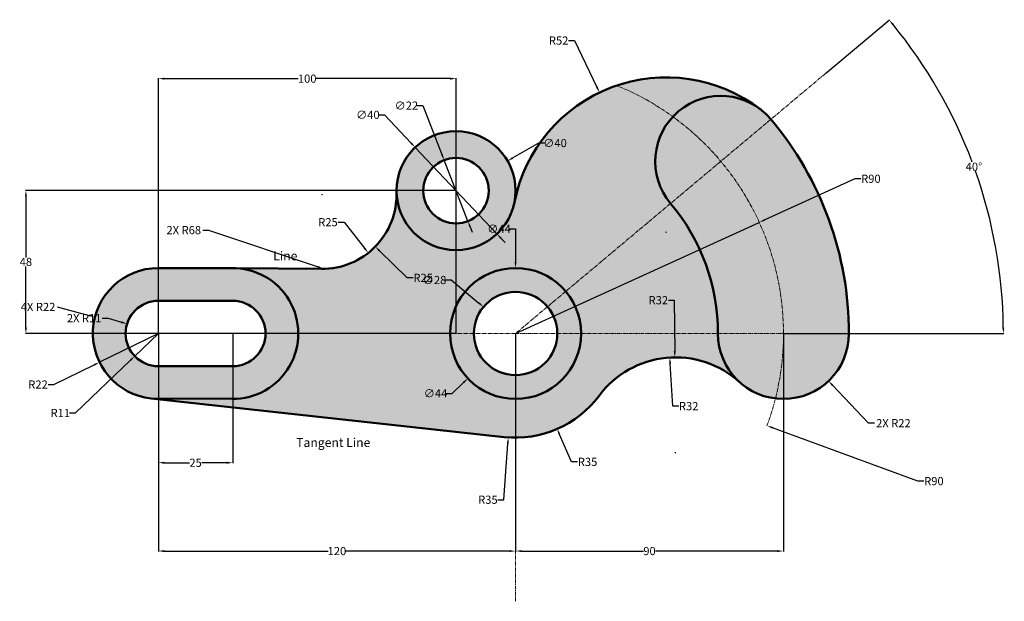
# Model space of a CAD drawing. Units: millimetres. Extents: x 249 to 580, y 179 to 375.
import ezdxf

# ---------------------------------------------------------------- set-up
doc = ezdxf.new("R2010")
doc.units = ezdxf.units.MM
doc.header["$MEASUREMENT"] = 0
doc.linetypes.add('CENTER', pattern=[2, 1.25, -0.25, 0.25, -0.25])
for name, color, linetype, lineweight in [('Dimensions', 20, 'Continuous', 25), ('M-CNTR', 251, 'CENTER', 18), ('M-HATC', 252, 'Continuous', 18), ('M-OUTL', 239, 'Continuous', 50), ('M-TEXT', 20, 'Continuous', 25)]:
    doc.layers.add(name, color=color, linetype=linetype, lineweight=lineweight)
doc.styles.get("Standard").update_dxf_attribs({"font": 'arial.ttf'})
doc.dimstyles.get("Standard").update_dxf_attribs({"dimtxt": 2.75, "dimasz": 2, "dimexe": 0.18, "dimexo": 0.0625, "dimgap": 0.09, "dimtad": 0, "dimtih": 1, "dimtoh": 1, "dimdec": 0, "dimzin": 0, "dimdsep": 46, "dimtxsty": 'Standard', "dimcen": 0.09, "dimadec": 0, "dimazin": 0, "dimtfac": 1, "dimtdec": 0, "dimtofl": 0, "dimtmove": 0, "dimatfit": 3, "dimfxl": 1, "dimtolj": 1, "dimtzin": 0, "dimarcsym": 0})

# ---------------------------------------------------------------- blocks, each defined once
blk = doc.blocks.new('*D1')
at = {"layer": 'Defpoints', "color": 0, "transparency": 16777216}
for p in [(295.42, 269.22), (320.42, 269.22), (320.42, 225.79)]:
    blk.add_point(p, dxfattribs=at)
at = {"layer": 'Dimensions', "color": 0, "lineweight": -2, "transparency": 16777216}
for p, q in [((295.42, 269.16), (295.42, 225.61)), ((320.42, 269.16), (320.42, 225.61)), ((297.42, 225.79), (305.83, 225.79)), ((318.42, 225.79), (310.01, 225.79))]:
    blk.add_line(p, q, dxfattribs=at)
at = {"layer": 'Dimensions', "color": 0, "transparency": 16777216}
for points in [[(297.42, 226.13), (297.42, 225.46), (295.42, 225.79)], [(318.42, 226.13), (318.42, 225.46), (320.42, 225.79)]]:
    blk.add_solid(points, dxfattribs=at)
at = {"layer": 'Dimensions', "color": 0, "transparency": 16777216, "insert": (307.92, 225.79), "char_height": 2.75, "attachment_point": 5}
blk.add_mtext('\\A1;25', dxfattribs=at)
blk = doc.blocks.new('*D2')
at = {"layer": 'Defpoints', "color": 0, "transparency": 16777216}
for p in [(295.42, 269.22), (415.42, 269.22), (415.42, 196.11)]:
    blk.add_point(p, dxfattribs=at)
at = {"layer": 'Dimensions', "color": 0, "lineweight": -2, "transparency": 16777216}
for p, q in [((295.42, 269.16), (295.42, 195.93)), ((415.42, 269.16), (415.42, 195.93)), ((297.42, 196.11), (352.43, 196.11)), ((413.42, 196.11), (358.41, 196.11))]:
    blk.add_line(p, q, dxfattribs=at)
at = {"layer": 'Dimensions', "color": 0, "transparency": 16777216}
for points in [[(297.42, 196.44), (297.42, 195.78), (295.42, 196.11)], [(413.42, 196.44), (413.42, 195.78), (415.42, 196.11)]]:
    blk.add_solid(points, dxfattribs=at)
at = {"layer": 'Dimensions', "color": 0, "transparency": 16777216, "insert": (355.42, 196.11), "char_height": 2.75, "attachment_point": 5}
blk.add_mtext('\\A1;120', dxfattribs=at)
blk = doc.blocks.new('*D3')
at = {"layer": 'Defpoints', "color": 0, "transparency": 16777216}
for p in [(295.42, 269.22), (287.48, 261.61)]:
    blk.add_point(p, dxfattribs=at)
at = {"layer": 'Dimensions', "color": 0, "lineweight": -2, "transparency": 16777216}
for p, q in [((295.42, 269.22), (287.48, 261.61)), ((267.59, 242.51), (286.04, 260.22)), ((265.59, 242.51), (267.59, 242.51))]:
    blk.add_line(p, q, dxfattribs=at)
at = {"layer": 'Dimensions', "color": 0, "transparency": 16777216}
blk.add_solid([(285.81, 260.46), (286.27, 259.98), (287.48, 261.61)], dxfattribs=at)
at = {"layer": 'Dimensions', "color": 0, "transparency": 16777216, "insert": (262.48, 242.51), "char_height": 2.75, "attachment_point": 5}
blk.add_mtext('\\A1;R11', dxfattribs=at)
blk = doc.blocks.new('*D4')
at = {"layer": 'Defpoints', "color": 0, "transparency": 16777216}
for p in [(295.42, 269.22), (275.66, 259.56)]:
    blk.add_point(p, dxfattribs=at)
at = {"layer": 'Dimensions', "color": 0, "lineweight": -2, "transparency": 16777216}
for p, q in [((295.42, 269.22), (275.66, 259.56)), ((260.35, 252.07), (273.86, 258.68)), ((258.35, 252.07), (260.35, 252.07))]:
    blk.add_line(p, q, dxfattribs=at)
at = {"layer": 'Dimensions', "color": 0, "transparency": 16777216}
blk.add_solid([(273.71, 258.98), (274.01, 258.38), (275.66, 259.56)], dxfattribs=at)
at = {"layer": 'Dimensions', "color": 0, "transparency": 16777216, "insert": (254.99, 252.07), "char_height": 2.75, "attachment_point": 5}
blk.add_mtext('\\A1;R22', dxfattribs=at)
blk = doc.blocks.new('*D5')
at = {"layer": 'Defpoints', "color": 0, "transparency": 16777216}
for p in [(350.44, 315.93), (365.94, 296.32)]:
    blk.add_point(p, dxfattribs=at)
at = {"layer": 'Dimensions', "color": 0, "lineweight": -2, "transparency": 16777216}
for p, q in [((355.8, 306.62), (357.8, 306.62)), ((357.8, 306.62), (364.7, 297.89))]:
    blk.add_line(p, q, dxfattribs=at)
at = {"layer": 'Dimensions', "color": 0, "transparency": 16777216}
blk.add_solid([(364.96, 298.09), (364.44, 297.68), (365.94, 296.32)], dxfattribs=at)
at = {"layer": 'Dimensions', "color": 0, "transparency": 16777216, "insert": (352.41, 306.62), "char_height": 2.75, "attachment_point": 5}
blk.add_mtext('\\A1;R25', dxfattribs=at)
blk = doc.blocks.new('*D6')
at = {"layer": 'Defpoints', "color": 0, "transparency": 16777216}
for p in [(391.43, 327.47), (399.41, 306.97)]:
    blk.add_point(p, dxfattribs=at)
at = {"layer": 'Dimensions', "color": 0, "lineweight": -2, "transparency": 16777216}
for p, q in [((382.28, 345.8), (384.28, 345.8)), ((384.28, 345.8), (390.7, 329.34)), ((399.41, 306.97), (391.43, 327.47)), ((400.14, 305.11), (400.86, 303.25))]:
    blk.add_line(p, q, dxfattribs=at)
at = {"layer": 'Dimensions', "color": 0, "transparency": 16777216}
for points in [[(391.01, 329.46), (390.39, 329.22), (391.43, 327.47)], [(400.45, 305.23), (399.83, 304.99), (399.41, 306.97)]]:
    blk.add_solid(points, dxfattribs=at)
at = {"layer": 'Dimensions', "color": 0, "transparency": 16777216, "insert": (378.74, 345.8), "char_height": 2.75, "attachment_point": 5}
blk.add_mtext('\\A1;∅22', dxfattribs=at)
blk = doc.blocks.new('*D7')
at = {"layer": 'Defpoints', "color": 0, "transparency": 16777216}
for p in [(381.69, 331.76), (409.15, 302.68)]:
    blk.add_point(p, dxfattribs=at)
at = {"layer": 'Dimensions', "color": 0, "lineweight": -2, "transparency": 16777216}
for p, q in [((369.36, 342.7), (371.36, 342.7)), ((371.36, 342.7), (380.32, 333.22)), ((409.15, 302.68), (381.69, 331.76)), ((410.52, 301.23), (411.9, 299.77))]:
    blk.add_line(p, q, dxfattribs=at)
at = {"layer": 'Dimensions', "color": 0, "transparency": 16777216}
for points in [[(380.56, 333.45), (380.07, 332.99), (381.69, 331.76)], [(410.77, 301.46), (410.28, 301), (409.15, 302.68)]]:
    blk.add_solid(points, dxfattribs=at)
at = {"layer": 'Dimensions', "color": 0, "transparency": 16777216, "insert": (365.81, 342.7), "char_height": 2.75, "attachment_point": 5}
blk.add_mtext('\\A1;∅40', dxfattribs=at)
blk = doc.blocks.new('*D8')
at = {"layer": 'Defpoints', "color": 0, "transparency": 16777216}
for p in [(395.42, 317.31), (250.92, 269.22), (395.42, 269.22)]:
    blk.add_point(p, dxfattribs=at)
at = {"layer": 'Dimensions', "color": 0, "lineweight": -2, "transparency": 16777216}
for p, q in [((395.36, 317.31), (250.74, 317.31)), ((250.92, 315.31), (250.92, 294.76)), ((250.92, 271.22), (250.92, 291.77)), ((395.36, 269.22), (250.74, 269.22))]:
    blk.add_line(p, q, dxfattribs=at)
at = {"layer": 'Dimensions', "color": 0, "transparency": 16777216}
for points in [[(250.58, 315.31), (251.25, 315.31), (250.92, 317.31)], [(250.58, 271.22), (251.25, 271.22), (250.92, 269.22)]]:
    blk.add_solid(points, dxfattribs=at)
at = {"layer": 'Dimensions', "color": 0, "transparency": 16777216, "insert": (250.92, 293.27), "char_height": 2.75, "attachment_point": 5}
blk.add_mtext('\\A1;48', dxfattribs=at)
blk = doc.blocks.new('*D9')
at = {"layer": 'Defpoints', "color": 0, "transparency": 16777216}
for p in [(443.61, 350.21), (466.06, 303.3)]:
    blk.add_point(p, dxfattribs=at)
at = {"layer": 'Dimensions', "color": 0, "lineweight": -2, "transparency": 16777216}
for p, q in [((433.26, 367.66), (435.26, 367.66)), ((435.26, 367.66), (442.75, 352.01)), ((465.97, 303.3), (466.15, 303.3)), ((466.06, 303.21), (466.06, 303.39))]:
    blk.add_line(p, q, dxfattribs=at)
at = {"layer": 'Dimensions', "color": 0, "transparency": 16777216}
blk.add_solid([(443.05, 352.16), (442.45, 351.87), (443.61, 350.21)], dxfattribs=at)
at = {"layer": 'Dimensions', "color": 0, "transparency": 16777216, "insert": (429.9, 367.66), "char_height": 2.75, "attachment_point": 5}
blk.add_mtext('\\A1;R52', dxfattribs=at)
blk = doc.blocks.new('*D10')
at = {"layer": 'Defpoints', "color": 0, "transparency": 16777216}
for p in [(467.23, 261.15), (469.16, 229.21)]:
    blk.add_point(p, dxfattribs=at)
at = {"layer": 'Dimensions', "color": 0, "lineweight": -2, "transparency": 16777216}
for p, q in [((468.22, 244.81), (467.35, 259.15)), ((470.22, 244.81), (468.22, 244.81))]:
    blk.add_line(p, q, dxfattribs=at)
at = {"layer": 'Dimensions', "color": 0, "transparency": 16777216}
blk.add_solid([(467.69, 259.17), (467.02, 259.13), (467.23, 261.15)], dxfattribs=at)
at = {"layer": 'Dimensions', "color": 0, "transparency": 16777216, "insert": (473.58, 244.81), "char_height": 2.75, "attachment_point": 5}
blk.add_mtext('\\A1;R32', dxfattribs=at)
blk = doc.blocks.new('*D11')
at = {"layer": 'Defpoints', "color": 0, "transparency": 16777216}
for p in [(415.42, 269.22), (429.41, 237.14)]:
    blk.add_point(p, dxfattribs=at)
at = {"layer": 'Dimensions', "color": 0, "lineweight": -2, "transparency": 16777216}
for p, q in [((415.33, 269.22), (415.51, 269.22)), ((415.42, 269.13), (415.42, 269.31)), ((434.23, 226.08), (430.21, 235.31)), ((436.23, 226.08), (434.23, 226.08))]:
    blk.add_line(p, q, dxfattribs=at)
at = {"layer": 'Dimensions', "color": 0, "transparency": 16777216}
blk.add_solid([(430.51, 235.44), (429.9, 235.17), (429.41, 237.14)], dxfattribs=at)
at = {"layer": 'Dimensions', "color": 0, "transparency": 16777216, "insert": (439.61, 226.08), "char_height": 2.75, "attachment_point": 5}
blk.add_mtext('\\A1;R35', dxfattribs=at)
blk = doc.blocks.new('*D12')
at = {"layer": 'Defpoints', "color": 0, "transparency": 16777216}
for p in [(519.45, 356.51), (574.88, 307.02), (415.42, 269.22), (415.42, 269.22), (505.42, 269.22)]:
    blk.add_point(p, dxfattribs=at)
at = {"layer": 'Dimensions', "color": 0, "lineweight": -2, "transparency": 16777216}
for p, q in [((519.5, 356.55), (541.1, 374.68)), ((505.48, 269.22), (579.48, 269.22))]:
    blk.add_line(p, q, dxfattribs=at)
for start, end in [(20.5569, 39.3008), (0.6992, 19.4451)]:
    blk.add_arc((415.42, 269.22), 163.88, start, end, dxfattribs=at)
at = {"layer": 'Dimensions', "color": 0, "transparency": 16777216}
for points in [[(541.98, 372.81), (542.49, 373.24), (540.96, 374.56)], [(579.62, 271.22), (578.95, 271.22), (579.3, 269.22)]]:
    blk.add_solid(points, dxfattribs=at)
at = {"layer": 'Dimensions', "color": 0, "transparency": 16777216, "insert": (569.42, 325.27), "char_height": 2.75, "attachment_point": 5}
blk.add_mtext('\\A1;40°', dxfattribs=at)
blk = doc.blocks.new('*D13')
at = {"layer": 'Defpoints', "color": 0, "transparency": 16777216}
for p in [(497.31, 306.57), (415.42, 269.22)]:
    blk.add_point(p, dxfattribs=at)
at = {"layer": 'Dimensions', "color": 0, "lineweight": -2, "transparency": 16777216}
for p, q in [((529.43, 321.22), (499.13, 307.4)), ((531.43, 321.22), (529.43, 321.22)), ((415.42, 269.22), (497.31, 306.57))]:
    blk.add_line(p, q, dxfattribs=at)
at = {"layer": 'Dimensions', "color": 0, "transparency": 16777216}
blk.add_solid([(498.99, 307.7), (499.26, 307.09), (497.31, 306.57)], dxfattribs=at)
at = {"layer": 'Dimensions', "color": 0, "transparency": 16777216, "insert": (534.8, 321.22), "char_height": 2.75, "attachment_point": 5}
blk.add_mtext('\\A1;R90', dxfattribs=at)
blk = doc.blocks.new('*D14')
at = {"layer": 'Defpoints', "color": 0, "transparency": 16777216}
for p in [(404.65, 278.17), (426.19, 260.28)]:
    blk.add_point(p, dxfattribs=at)
at = {"layer": 'Dimensions', "color": 0, "lineweight": -2, "transparency": 16777216}
for p, q in [((391.77, 287.2), (393.77, 287.2)), ((393.77, 287.2), (403.11, 279.44)), ((415.33, 269.22), (415.51, 269.22)), ((415.42, 269.13), (415.42, 269.31))]:
    blk.add_line(p, q, dxfattribs=at)
at = {"layer": 'Dimensions', "color": 0, "transparency": 16777216}
blk.add_solid([(403.32, 279.7), (402.9, 279.19), (404.65, 278.17)], dxfattribs=at)
at = {"layer": 'Dimensions', "color": 0, "transparency": 16777216, "insert": (388.21, 287.2), "char_height": 2.75, "attachment_point": 5}
blk.add_mtext('\\A1;∅28', dxfattribs=at)
blk = doc.blocks.new('*D15')
at = {"layer": 'Defpoints', "color": 0, "transparency": 16777216}
for p in [(431.42, 284.32), (399.42, 254.13)]:
    blk.add_point(p, dxfattribs=at)
at = {"layer": 'Dimensions', "color": 0, "lineweight": -2, "transparency": 16777216}
for p, q in [((415.33, 269.22), (415.51, 269.22)), ((415.42, 269.13), (415.42, 269.31)), ((394.1, 249.11), (397.96, 252.76)), ((392.1, 249.11), (394.1, 249.11))]:
    blk.add_line(p, q, dxfattribs=at)
at = {"layer": 'Dimensions', "color": 0, "transparency": 16777216}
blk.add_solid([(397.73, 253), (398.19, 252.51), (399.42, 254.13)], dxfattribs=at)
at = {"layer": 'Dimensions', "color": 0, "transparency": 16777216, "insert": (388.55, 249.11), "char_height": 2.75, "attachment_point": 5}
blk.add_mtext('\\A1;∅44', dxfattribs=at)
blk = doc.blocks.new('*D16')
at = {"layer": 'Defpoints', "color": 0, "transparency": 16777216}
for p in [(415.42, 269.22), (505.42, 269.22), (505.42, 196.11)]:
    blk.add_point(p, dxfattribs=at)
at = {"layer": 'Dimensions', "color": 0, "lineweight": -2, "transparency": 16777216}
for p, q in [((415.42, 269.16), (415.42, 195.93)), ((505.42, 269.16), (505.42, 195.93)), ((417.42, 196.11), (458.36, 196.11)), ((503.42, 196.11), (462.47, 196.11))]:
    blk.add_line(p, q, dxfattribs=at)
at = {"layer": 'Dimensions', "color": 0, "transparency": 16777216}
for points in [[(417.42, 196.44), (417.42, 195.78), (415.42, 196.11)], [(503.42, 196.44), (503.42, 195.78), (505.42, 196.11)]]:
    blk.add_solid(points, dxfattribs=at)
at = {"layer": 'Dimensions', "color": 0, "transparency": 16777216, "insert": (460.42, 196.11), "char_height": 2.75, "attachment_point": 5}
blk.add_mtext('\\A1;90', dxfattribs=at)
blk = doc.blocks.new('*D17')
at = {"layer": 'Defpoints', "color": 0, "transparency": 16777216}
for p in [(505.42, 269.22), (520.56, 253.27)]:
    blk.add_point(p, dxfattribs=at)
at = {"layer": 'Dimensions', "color": 0, "lineweight": -2, "transparency": 16777216}
for p, q in [((505.33, 269.22), (505.51, 269.22)), ((505.42, 269.13), (505.42, 269.31)), ((534.03, 239.08), (521.94, 251.82)), ((536.03, 239.08), (534.03, 239.08))]:
    blk.add_line(p, q, dxfattribs=at)
at = {"layer": 'Dimensions', "color": 0, "transparency": 16777216}
blk.add_solid([(522.18, 252.04), (521.7, 251.59), (520.56, 253.27)], dxfattribs=at)
at = {"layer": 'Dimensions', "color": 0, "transparency": 16777216, "insert": (542.37, 239.08), "char_height": 2.75, "attachment_point": 5}
blk.add_mtext('\\A1;2X R22', dxfattribs=at)
blk = doc.blocks.new('*D18')
at = {"layer": 'Defpoints', "color": 0, "transparency": 16777216}
for p in [(395.42, 354.87), (295.42, 269.22), (395.42, 269.22)]:
    blk.add_point(p, dxfattribs=at)
at = {"layer": 'Dimensions', "color": 0, "lineweight": -2, "transparency": 16777216}
for p, q in [((295.42, 269.29), (295.42, 355.05)), ((297.42, 354.87), (342.43, 354.87)), ((393.42, 354.87), (348.41, 354.87)), ((395.42, 269.29), (395.42, 355.05))]:
    blk.add_line(p, q, dxfattribs=at)
at = {"layer": 'Dimensions', "color": 0, "transparency": 16777216}
for points in [[(297.42, 355.2), (297.42, 354.53), (295.42, 354.87)], [(393.42, 355.2), (393.42, 354.53), (395.42, 354.87)]]:
    blk.add_solid(points, dxfattribs=at)
at = {"layer": 'Dimensions', "color": 0, "transparency": 16777216, "insert": (345.42, 354.87), "char_height": 2.75, "attachment_point": 5}
blk.add_mtext('\\A1;100', dxfattribs=at)
blk = doc.blocks.new('*D19')
at = {"layer": 'Defpoints', "color": 0, "transparency": 16777216}
for p in [(415.42, 269.22), (499.91, 238.22)]:
    blk.add_point(p, dxfattribs=at)
at = {"layer": 'Dimensions', "color": 0, "lineweight": -2, "transparency": 16777216}
for p, q in [((415.33, 269.22), (415.51, 269.22)), ((415.42, 269.13), (415.42, 269.31)), ((550.6, 219.61), (501.79, 237.53)), ((552.6, 219.61), (550.6, 219.61))]:
    blk.add_line(p, q, dxfattribs=at)
at = {"layer": 'Dimensions', "color": 0, "transparency": 16777216}
blk.add_solid([(501.9, 237.84), (501.67, 237.21), (499.91, 238.22)], dxfattribs=at)
at = {"layer": 'Dimensions', "color": 0, "transparency": 16777216, "insert": (555.97, 219.61), "char_height": 2.75, "attachment_point": 5}
blk.add_mtext('\\A1;R90', dxfattribs=at)
blk = doc.blocks.new('*D20')
at = {"layer": 'Defpoints', "color": 0, "transparency": 16777216}
for p in [(350.98, 290.93), (415.42, 269.22)]:
    blk.add_point(p, dxfattribs=at)
at = {"layer": 'Dimensions', "color": 0, "lineweight": -2, "transparency": 16777216}
for p, q in [((310.31, 303.96), (312.31, 303.96)), ((312.31, 303.96), (349.08, 291.57)), ((415.33, 269.22), (415.51, 269.22)), ((415.42, 269.13), (415.42, 269.31))]:
    blk.add_line(p, q, dxfattribs=at)
at = {"layer": 'Dimensions', "color": 0, "transparency": 16777216}
blk.add_solid([(349.19, 291.89), (348.98, 291.26), (350.98, 290.93)], dxfattribs=at)
at = {"layer": 'Dimensions', "color": 0, "transparency": 16777216, "insert": (303.96, 303.96), "char_height": 2.75, "attachment_point": 5}
blk.add_mtext('\\A1;2X R68', dxfattribs=at)
blk = doc.blocks.new('*D21')
at = {"layer": 'Defpoints', "color": 0, "transparency": 16777216}
for p in [(415.42, 269.22), (412.98, 234.31)]:
    blk.add_point(p, dxfattribs=at)
at = {"layer": 'Dimensions', "color": 0, "lineweight": -2, "transparency": 16777216}
for p, q in [((415.33, 269.22), (415.51, 269.22)), ((415.42, 269.13), (415.42, 269.31)), ((411.52, 213.36), (412.84, 232.31)), ((409.52, 213.36), (411.52, 213.36))]:
    blk.add_line(p, q, dxfattribs=at)
at = {"layer": 'Dimensions', "color": 0, "transparency": 16777216}
blk.add_solid([(412.51, 232.34), (413.17, 232.29), (412.98, 234.31)], dxfattribs=at)
at = {"layer": 'Dimensions', "color": 0, "transparency": 16777216, "insert": (406.13, 213.36), "char_height": 2.75, "attachment_point": 5}
blk.add_mtext('\\A1;R35', dxfattribs=at)
blk = doc.blocks.new('*D22')
at = {"layer": 'Defpoints', "color": 0, "transparency": 16777216}
for p in [(350.44, 315.93), (368.28, 298.42)]:
    blk.add_point(p, dxfattribs=at)
at = {"layer": 'Dimensions', "color": 0, "lineweight": -2, "transparency": 16777216}
for p, q in [((350.35, 315.93), (350.53, 315.93)), ((350.44, 315.84), (350.44, 316.02)), ((378.99, 287.92), (369.71, 297.02)), ((380.99, 287.92), (378.99, 287.92))]:
    blk.add_line(p, q, dxfattribs=at)
at = {"layer": 'Dimensions', "color": 0, "transparency": 16777216}
blk.add_solid([(369.94, 297.26), (369.48, 296.79), (368.28, 298.42)], dxfattribs=at)
at = {"layer": 'Dimensions', "color": 0, "transparency": 16777216, "insert": (384.37, 287.92), "char_height": 2.75, "attachment_point": 5}
blk.add_mtext('\\A1;R25', dxfattribs=at)
blk = doc.blocks.new('*D23')
at = {"layer": 'Defpoints', "color": 0, "transparency": 16777216}
for p in [(274.14, 274.8), (295.42, 269.22)]:
    blk.add_point(p, dxfattribs=at)
at = {"layer": 'Dimensions', "color": 0, "lineweight": -2, "transparency": 16777216}
for p, q in [((261.37, 278.15), (272.2, 275.31)), ((295.33, 269.22), (295.51, 269.22)), ((295.42, 269.13), (295.42, 269.31))]:
    blk.add_line(p, q, dxfattribs=at)
at = {"layer": 'Dimensions', "color": 0, "transparency": 16777216}
blk.add_solid([(272.29, 275.63), (272.12, 274.99), (274.14, 274.8)], dxfattribs=at)
at = {"layer": 'Dimensions', "color": 0, "transparency": 16777216, "insert": (255, 278.15), "char_height": 2.75, "attachment_point": 5}
blk.add_mtext('\\A1;4X R22', dxfattribs=at)
blk = doc.blocks.new('*D24')
at = {"layer": 'Defpoints', "color": 0, "transparency": 16777216}
for p in [(415.42, 291.22), (415.42, 247.22)]:
    blk.add_point(p, dxfattribs=at)
at = {"layer": 'Dimensions', "color": 0, "lineweight": -2, "transparency": 16777216}
for p, q in [((413.42, 304.42), (415.42, 304.42)), ((415.42, 304.42), (415.42, 293.22)), ((415.33, 269.22), (415.51, 269.22)), ((415.42, 269.13), (415.42, 269.31))]:
    blk.add_line(p, q, dxfattribs=at)
at = {"layer": 'Dimensions', "color": 0, "transparency": 16777216}
blk.add_solid([(415.75, 293.22), (415.09, 293.22), (415.42, 291.22)], dxfattribs=at)
at = {"layer": 'Dimensions', "color": 0, "transparency": 16777216, "insert": (409.87, 304.42), "char_height": 2.75, "attachment_point": 5}
blk.add_mtext('\\A1;∅44', dxfattribs=at)
blk = doc.blocks.new('*D25')
at = {"layer": 'Defpoints', "color": 0, "transparency": 16777216}
for p in [(412.74, 327.22), (378.1, 307.22)]:
    blk.add_point(p, dxfattribs=at)
at = {"layer": 'Dimensions', "color": 0, "lineweight": -2, "transparency": 16777216}
for p, q in [((423.13, 333.22), (414.47, 328.22)), ((425.13, 333.22), (423.13, 333.22)), ((395.33, 317.22), (395.51, 317.22)), ((395.42, 317.13), (395.42, 317.31))]:
    blk.add_line(p, q, dxfattribs=at)
at = {"layer": 'Dimensions', "color": 0, "transparency": 16777216}
blk.add_solid([(414.31, 328.51), (414.64, 327.93), (412.74, 327.22)], dxfattribs=at)
at = {"layer": 'Dimensions', "color": 0, "transparency": 16777216, "insert": (428.68, 333.22), "char_height": 2.75, "attachment_point": 5}
blk.add_mtext('\\A1;∅40', dxfattribs=at)
blk = doc.blocks.new('*D26')
at = {"layer": 'Defpoints', "color": 0, "transparency": 16777216}
for p in [(284.9, 272.44), (295.42, 269.22)]:
    blk.add_point(p, dxfattribs=at)
at = {"layer": 'Dimensions', "color": 0, "lineweight": -2, "transparency": 16777216}
for p, q in [((276.59, 274.37), (278.59, 274.37)), ((278.59, 274.37), (282.99, 273.02)), ((295.33, 269.22), (295.51, 269.22)), ((295.42, 269.13), (295.42, 269.31))]:
    blk.add_line(p, q, dxfattribs=at)
at = {"layer": 'Dimensions', "color": 0, "transparency": 16777216}
blk.add_solid([(283.09, 273.34), (282.89, 272.71), (284.9, 272.44)], dxfattribs=at)
at = {"layer": 'Dimensions', "color": 0, "transparency": 16777216, "insert": (270.5, 274.37), "char_height": 2.75, "attachment_point": 5}
blk.add_mtext('\\A1;2X R11', dxfattribs=at)
blk = doc.blocks.new('*D27')
at = {"layer": 'Defpoints', "color": 0, "transparency": 16777216}
for p in [(468.9, 261.21), (469.16, 229.21)]:
    blk.add_point(p, dxfattribs=at)
at = {"layer": 'Dimensions', "color": 0, "lineweight": -2, "transparency": 16777216}
for p, q in [((466.75, 280.41), (468.75, 280.41)), ((468.75, 280.41), (468.88, 263.21)), ((469.07, 229.21), (469.25, 229.21)), ((469.16, 229.12), (469.16, 229.3))]:
    blk.add_line(p, q, dxfattribs=at)
at = {"layer": 'Dimensions', "color": 0, "transparency": 16777216}
blk.add_solid([(469.22, 263.21), (468.55, 263.21), (468.9, 261.21)], dxfattribs=at)
at = {"layer": 'Dimensions', "color": 0, "transparency": 16777216, "insert": (463.38, 280.41), "char_height": 2.75, "attachment_point": 5}
blk.add_mtext('\\A1;R32', dxfattribs=at)

msp = doc.modelspace()

# ---------------------------------------------------------------- hatches: boundary and pattern name
at = {"layer": 'M-HATC'}
h = msp.add_hatch(color=256, dxfattribs=at)
h.dxf.hatch_style = 1
h.paths.add_polyline_path([(467.51, 312.93), (432.27, 283.36, -0.176327), (437.42, 269.22), (483.42, 269.22, 0.176327)])
h.paths.add_polyline_path([(467.51, 312.93, -0.378764), (468.27, 342.07, 0.060186), (449.4, 352.56, 0.26872), (415.04, 313.36, -0.894189), (375.43, 316.65, -0.416255), (350.98, 290.94, 0.000048), (350.98, 290.93), (320.85, 291.22, -0.408552), (342.42, 269.22), (393.42, 269.22, -0.700208), (432.27, 283.36)])
h.paths.add_polyline_path([(449.4, 352.56, -0.060186), (468.27, 342.07, -0.386948), (497.78, 344.51, 0.250642)])
h.paths.add_polyline_path([(393.42, 269.22), (342.42, 269.22, -0.414214), (320.42, 247.22), (293.04, 247.35), (411.63, 234.43, 0.027143), (415.42, 234.22), (415.42, 247.22, -0.414214)])
h.paths.add_polyline_path([(490.65, 252.92, -0.211722), (483.42, 269.22), (437.42, 269.22, -0.414214), (415.42, 247.22), (415.42, 234.22, 0.236982), (443.49, 248.32, -0.442678)])
h = msp.add_hatch(color=256, dxfattribs=at)
h.dxf.hatch_style = 1
h.paths.add_polyline_path([(320.85, 291.22), (295.42, 291.22, 0.414214), (273.42, 269.22), (284.42, 269.22, -0.414214), (295.42, 280.22), (320.42, 280.22, -0.414214), (331.42, 269.22), (342.42, 269.22, 0.408552)])
h.paths.add_polyline_path([(342.42, 269.22), (331.42, 269.22, -0.414214), (320.42, 258.22), (295.42, 258.22, -0.414214), (284.42, 269.22), (273.42, 269.22, 0.382767), (293.04, 247.35), (320.42, 247.22, 0.414214)])
h.paths.add_polyline_path([(415.42, 317.22, 1), (375.42, 317.22, 1)])
h.paths.add_polyline_path([(384.42, 317.22, -1), (406.42, 317.22, -1)], flags=16)
h.paths.add_polyline_path([(393.42, 269.22), (401.42, 269.22, -0.700208), (426.14, 278.22), (432.27, 283.36, 0.700208)])
h.paths.add_polyline_path([(432.27, 283.36), (426.14, 278.22, -0.176327), (429.42, 269.22), (437.42, 269.22, 0.176327)])
h.paths.add_polyline_path([(437.42, 269.22), (429.42, 269.22, -0.414214), (415.42, 255.22), (415.42, 247.22, 0.414214)])
h.paths.add_polyline_path([(415.42, 255.22, -0.414214), (401.42, 269.22), (393.42, 269.22, 0.414214), (415.42, 247.22)])
h.paths.add_polyline_path([(501.22, 341.22, 0.450574), (468.27, 342.07, -0.061341), (484.36, 327.07)])
h.paths.add_polyline_path([(468.27, 342.07, 0.378764), (467.51, 312.93), (484.36, 327.07, 0.061341)])
h.paths.add_polyline_path([(527.42, 269.22), (505.42, 269.22, -0.061341), (502.73, 247.39, 0.450574)])
h.paths.add_polyline_path([(505.42, 269.22), (483.42, 269.22, 0.378764), (502.73, 247.39, 0.061341)])
h.paths.add_polyline_path([(501.22, 341.22), (484.36, 327.07, -0.176327), (505.42, 269.22), (527.42, 269.22, 0.176327)])
h.paths.add_polyline_path([(484.36, 327.07), (467.51, 312.93, -0.176327), (483.42, 269.22), (505.34, 269.22, 0.000613), (505.42, 269.32, 0.176051)])

# ---------------------------------------------------------------- linework, layer by layer
at = {"layer": 'M-CNTR'}
for points in [[(519.45, 356.51), (415.42, 269.22), (320.42, 269.22), (295.42, 269.22), (258.53, 269.22)], [(415.42, 179.22), (415.42, 269.22), (505.42, 269.22), (575.56, 269.22)]]:
    msp.add_lwpolyline(points, dxfattribs=at)
msp.add_arc((415.42, 269.22), 90, 339.8012, 67.8178, dxfattribs=at)
at = {"layer": 'M-OUTL'}
for p, q in [((295.42, 291.22), (320.85, 291.22)), ((320.42, 291.22), (350.98, 290.93)), ((295.42, 280.22), (320.42, 280.22)), ((295.42, 258.22), (320.42, 258.22)), ((293.04, 247.35), (411.63, 234.43)), ((293.04, 247.35), (320.42, 247.22))]:
    msp.add_line(p, q, dxfattribs=at)
for centre, radius in [((395.42, 317.22), 20), ((395.42, 317.22), 11), ((415.42, 269.22), 22), ((415.42, 269.22), 14)]:
    msp.add_circle(centre, radius, dxfattribs=at)
for centre, radius, start, end in [((466.06, 303.3), 52, 52.405, 168.8531), ((484.36, 327.07), 22, 40, 220), ((415.42, 269.22), 112, 0, 40), ((350.44, 315.93), 25, 269.4451, 1.6421), ((415.42, 269.22), 68, 0, 40), ((295.42, 269.22), 22, 89.9814, 263.7808), ((320.42, 269.22), 22, 269.4582, 91.0912), ((415.42, 269.22), 68, 161.3759, 161.3868), ((295.42, 269.22), 11, 90, 270), ((320.42, 269.22), 11, 270, 90), ((505.42, 269.22), 22, 180, 0), ((466.06, 303.3), 52, 319.0503, 319.1907), ((469.16, 229.21), 32, 47.8169, 143.3285), ((415.42, 269.22), 35, 263.7808, 323.3285)]:
    msp.add_arc(centre, radius, start, end, dxfattribs=at)

# ---------------------------------------------------------------- texts
at = {"layer": 'M-TEXT', "char_height": 3, "attachment_point": 1}
for s, width, insert in [('Line', 16.77, (334.02, 296.8)), ('Tangent Line', 40.3099, (341.74, 234.09))]:
    msp.add_mtext_dynamic_manual_height_columns(s, width=width, gutter_width=1, heights=[0], dxfattribs=dict(at, insert=insert))

# ---------------------------------------------------------------- dimensions: what is measured, and where the dimension line sits
at = {"layer": 'Dimensions'}
dim = msp.add_angular_dim_2l(base=(574.88, 307.02), line1=((415.42, 269.22), (505.42, 269.22)), line2=((519.45, 356.51), (415.42, 269.22)), dimstyle='Standard', override={"dimclrd": 0, "dimclre": 0, "dimclrt": 0}, dxfattribs=at)
dim.commit()
dim.dimension.update_dxf_attribs({"geometry": '*D12', "text_midpoint": (569.42, 325.27), "dimtype": 162})
for center, mpoint, override, picture, middle in [((466.06, 303.3), (443.61, 350.21), {"dimclrd": 0, "dimclre": 0, "dimclrt": 0}, '*D9', (429.9, 367.66)), ((415.42, 269.22), (497.31, 306.57), {"dimclrd": 0, "dimclre": 0, "dimclrt": 0, "dimtofl": 1}, '*D13', (534.8, 321.22)), ((350.44, 315.93), (365.94, 296.32), {"dimclrd": 0, "dimclre": 0, "dimclrt": 0}, '*D5', (352.41, 306.62)), ((350.44, 315.93), (368.28, 298.42), {"dimdec": 0, "dimlfac": 1, "dimrnd": 0, "dimzin": 0, "dimdsep": 46, "dimlunit": 2}, '*D22', (384.37, 287.92)), ((469.16, 229.21), (468.9, 261.21), {"dimdec": 0, "dimlfac": 1, "dimrnd": 0, "dimzin": 0, "dimdsep": 46, "dimlunit": 2}, '*D27', (463.38, 280.41)), ((295.42, 269.22), (275.66, 259.56), {"dimclrd": 0, "dimclre": 0, "dimclrt": 0, "dimtofl": 1}, '*D4', (254.99, 252.07)), ((295.42, 269.22), (287.48, 261.61), {"dimclrd": 0, "dimclre": 0, "dimclrt": 0, "dimtofl": 1}, '*D3', (262.48, 242.51)), ((415.42, 269.22), (412.98, 234.31), {"dimdec": 0, "dimlfac": 1, "dimrnd": 0, "dimzin": 0, "dimdsep": 46, "dimlunit": 2}, '*D21', (406.13, 213.36)), ((415.42, 269.22), (429.41, 237.14), {"dimclrd": 0, "dimclre": 0, "dimclrt": 0}, '*D11', (439.61, 226.08)), ((415.42, 269.22), (499.91, 238.22), {"dimdec": 0, "dimlfac": 1, "dimrnd": 0, "dimzin": 0, "dimdsep": 46, "dimlunit": 2}, '*D19', (555.97, 219.61)), ((469.16, 229.21), (467.23, 261.15), {"dimclrd": 0, "dimclre": 0, "dimclrt": 0}, '*D10', (473.58, 244.81))]:
    dim = msp.add_radius_dim(center=center, mpoint=mpoint, dimstyle='Standard', override=override, dxfattribs=at)
    dim.commit()
    dim.dimension.update_dxf_attribs({"geometry": picture, "text_midpoint": middle, "dimtype": 164})
dim = msp.add_linear_dim(base=(395.42, 354.87), p1=(295.42, 269.22), p2=(395.42, 269.22), dimstyle='Standard', override={"dimclrd": 0, "dimclre": 0, "dimclrt": 0}, dxfattribs=at)
dim.commit()
dim.dimension.update_dxf_attribs({"geometry": '*D18', "text_midpoint": (345.42, 354.87), "dimtype": 160})
for p1, p2, override, picture, middle in [((399.41, 306.97), (391.43, 327.47), {"dimclrd": 0, "dimclre": 0, "dimclrt": 0, "dimtofl": 1}, '*D6', (378.74, 345.8)), ((409.15, 302.68), (381.69, 331.76), {"dimclrd": 0, "dimclre": 0, "dimclrt": 0, "dimtofl": 1}, '*D7', (365.81, 342.7)), ((378.1, 307.22), (412.74, 327.22), {"dimdec": 0, "dimlfac": 1, "dimrnd": 0, "dimzin": 0, "dimdsep": 46, "dimlunit": 2}, '*D25', (428.68, 333.22)), ((415.42, 247.22), (415.42, 291.22), {"dimdec": 0, "dimlfac": 1, "dimrnd": 0, "dimzin": 0, "dimdsep": 46, "dimlunit": 2}, '*D24', (409.87, 304.42)), ((426.19, 260.28), (404.65, 278.17), {"dimclrd": 0, "dimclre": 0, "dimclrt": 0}, '*D14', (388.21, 287.2)), ((431.42, 284.32), (399.42, 254.13), {"dimclrd": 0, "dimclre": 0, "dimclrt": 0}, '*D15', (388.55, 249.11))]:
    dim = msp.add_diameter_dim_2p(p1=p1, p2=p2, dimstyle='Standard', override=override, dxfattribs=at)
    dim.commit()
    dim.dimension.update_dxf_attribs({"geometry": picture, "text_midpoint": middle, "dimtype": 163})
dim = msp.add_linear_dim(base=(250.92, 269.22), p1=(395.42, 317.31), p2=(395.42, 269.22), angle=90, dimstyle='Standard', override={"dimclrd": 0, "dimclre": 0, "dimclrt": 0}, dxfattribs=at)
dim.commit()
dim.dimension.update_dxf_attribs({"geometry": '*D8', "text_midpoint": (250.92, 293.27)})
for center, mpoint, text, override, picture, middle in [((415.42, 269.22), (350.98, 290.93), '2X <>', {"dimdec": 0, "dimlfac": 1, "dimrnd": 0, "dimzin": 0, "dimdsep": 46, "dimlunit": 2}, '*D20', (303.96, 303.96)), ((295.42, 269.22), (274.14, 274.8), '4X <>', {"dimdec": 0, "dimlfac": 1, "dimrnd": 0, "dimzin": 0, "dimdsep": 46, "dimlunit": 2}, '*D23', (261.37, 278.15)), ((295.42, 269.22), (284.9, 272.44), '2X <>', {"dimdec": 0, "dimlfac": 1, "dimrnd": 0, "dimzin": 0, "dimdsep": 46, "dimlunit": 2}, '*D26', (270.5, 274.37)), ((505.42, 269.22), (520.56, 253.27), '2X R22', {"dimclrd": 0, "dimclre": 0, "dimclrt": 0}, '*D17', (542.37, 239.08))]:
    dim = msp.add_radius_dim(center=center, mpoint=mpoint, text=text, dimstyle='Standard', override=override, dxfattribs=at)
    dim.commit()
    dim.dimension.update_dxf_attribs({"geometry": picture, "text_midpoint": middle, "dimtype": 164})
for base, p1, p2, picture, middle in [((320.42, 225.79), (295.42, 269.22), (320.42, 269.22), '*D1', (307.92, 225.79)), ((415.42, 196.11), (295.42, 269.22), (415.42, 269.22), '*D2', (355.42, 196.11)), ((505.42, 196.11), (415.42, 269.22), (505.42, 269.22), '*D16', (460.42, 196.11))]:
    dim = msp.add_linear_dim(base=base, p1=p1, p2=p2, dimstyle='Standard', override={"dimclrd": 0, "dimclre": 0, "dimclrt": 0}, dxfattribs=at)
    dim.commit()
    dim.dimension.update_dxf_attribs({"geometry": picture, "text_midpoint": middle})

doc.saveas('drawing.dxf')
